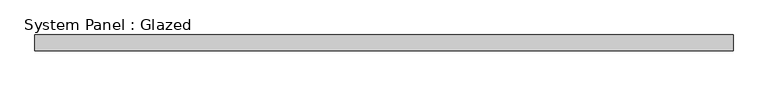
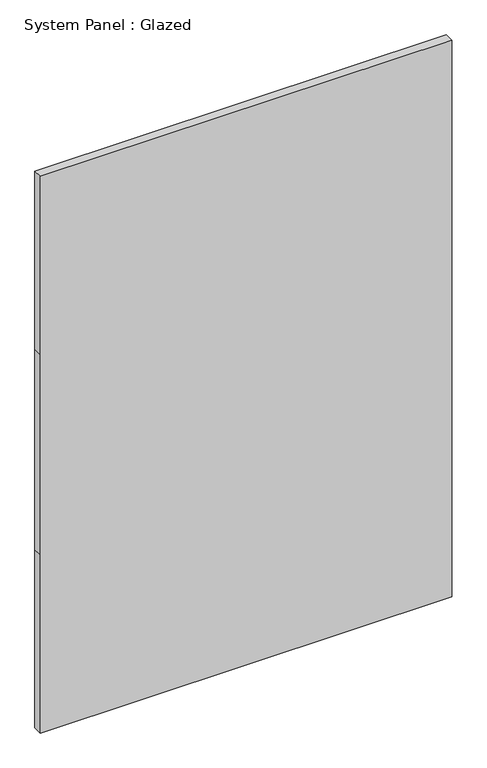
"""IFC4 building model written with IfcOpenShell, lengths in millimetres: plate geometry, System Panel : Glazed."""

from ifc_helpers import new_model, si_unit, frame, origin, place, context, project, spatial, polyline, outline, extrude, source, transform, mapped, element, save


def system_panel_glazed_5b59eb94(model_context):
    return source(origin(), model_context, "Body", "SweptSolid", [
        extrude(outline(polyline([(0.0, -568.325), (0.0, 568.325), (520.7173759, 568.325), (1104.9347517, 568.325), (1625.6521276, 568.325), (1625.6521276, -568.325), (1104.9347517, -568.325), (520.7173759, -568.325), (0.0, -568.325)])), frame((0.0, 19.05, 0.0), z_axis=(0.0, 1.0, 0.0), x_axis=(0.0, 0.0, 1.0)), (0.0, 0.0, 1.0), 25.4),
    ])


if __name__ == "__main__":
    model = new_model("IFC4")
    model_context = context("Model", 3, world=origin())
    ifc_project = project(units=[si_unit("LENGTHUNIT", "METRE", prefix="MILLI")], contexts=[model_context])
    site = spatial("IfcSite", under=ifc_project)
    building = spatial("IfcBuilding", under=site)
    placement = place(None, origin())
    system_panel_glazed_shape = system_panel_glazed_5b59eb94(model_context)
    element("IfcPlate", 1, ObjectType="System Panel : Glazed", at=placement, inside=building, context=model_context, shape_type="MappedRepresentation", body=[
        mapped(system_panel_glazed_shape, transform((0.0, 0.0, 0.0), x_axis=(1.0, 0.0, 0.0), y_axis=(0.0, 1.0, 0.0), z_axis=(0.0, 0.0, 1.0))),
    ])
    save(model, "model.ifc")

# Revit data of these elements
# Type "System Panel : Glazed"
#   Construction Type Id = "GSP4R"
#   Analytic Construction = "1/8 in Pilkington single glazing"
#   Visual Light Transmittance = 0.9
#   Solar Heat Gain Coefficient = 0.86
#   Heat Transfer Coefficient (U) = 1.18115 BTU/(h·ft²·°F)
#   Define Thermal Properties by = 1
# Element 1 (IfcPlate, "System Panel : Glazed")
#   Materials on its faces: "Glass"
# Materials
#   "Glass": class "Glass", colour RGB 0 128 192, transparency 0.75, Description = "Soda Lime Glass", Cost = 0
